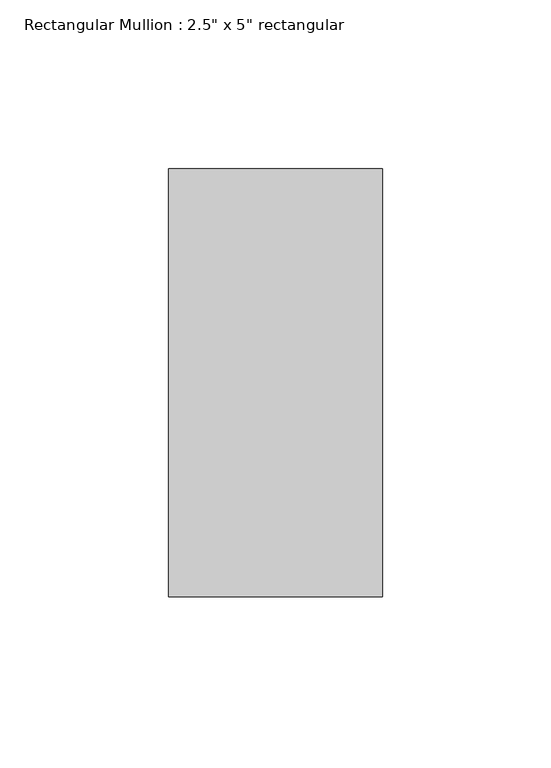
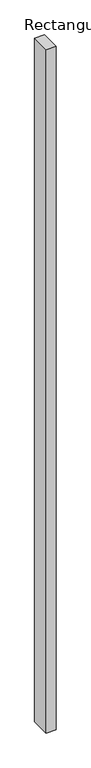
"""IFC4 building model written with IfcOpenShell, lengths in millimetres: member geometry."""

from ifc_helpers import new_model, si_unit, frame, origin, place, context, project, spatial, polyline, outline, extrude, source, transform, mapped, element, save


def member_6d14b308(model_context):
    return source(origin(), model_context, "Body", "SweptSolid", [
        extrude(outline(polyline([(0.0, 63.5), (0.0, -63.5), (-63.5, -63.5), (-63.5, 63.5), (0.0, 63.5)])), frame((0.0, 0.0, -4648.2), z_axis=(0.0, 0.0, 1.0), x_axis=(1.0, 0.0, 0.0)), (0.0, 0.0, 1.0), 4648.2),
    ])


if __name__ == "__main__":
    model = new_model("IFC4")
    model_context = context("Model", 3, world=origin())
    ifc_project = project(units=[si_unit("LENGTHUNIT", "METRE", prefix="MILLI")], contexts=[model_context])
    site = spatial("IfcSite", under=ifc_project)
    building = spatial("IfcBuilding", under=site)
    placement = place(None, origin())
    member_shape = member_6d14b308(model_context)
    element("IfcMember", 1, ObjectType="Rectangular Mullion : 2.5\" x 5\" rectangular", at=placement, inside=building, context=model_context, shape_type="MappedRepresentation", body=[
        mapped(member_shape, transform((0.0, 0.0, 0.0), x_axis=(1.0, 0.0, 0.0), y_axis=(0.0, 1.0, 0.0), z_axis=(0.0, 0.0, 1.0))),
    ])
    save(model, "model.ifc")

# Revit data of these elements
# Type "Rectangular Mullion : 2.5\" x 5\" rectangular"
#   built-in parameter 1007304 = 0.416667 (stored number, unit not read)
#   built-in parameter 1007301 = 0.104167 (stored number, unit not read)
#   built-in parameter 1007300 = 0.104167 (stored number, unit not read)
# Element 1 (IfcMember, "Rectangular Mullion : 2.5\" x 5\" rectangular")
#   Materials on its faces: "Aluminum"
# Materials
#   "Aluminum": class "Metal", colour RGB 247 247 247, transparency 0, Description = "Aluminum 6061", Cost = 0
